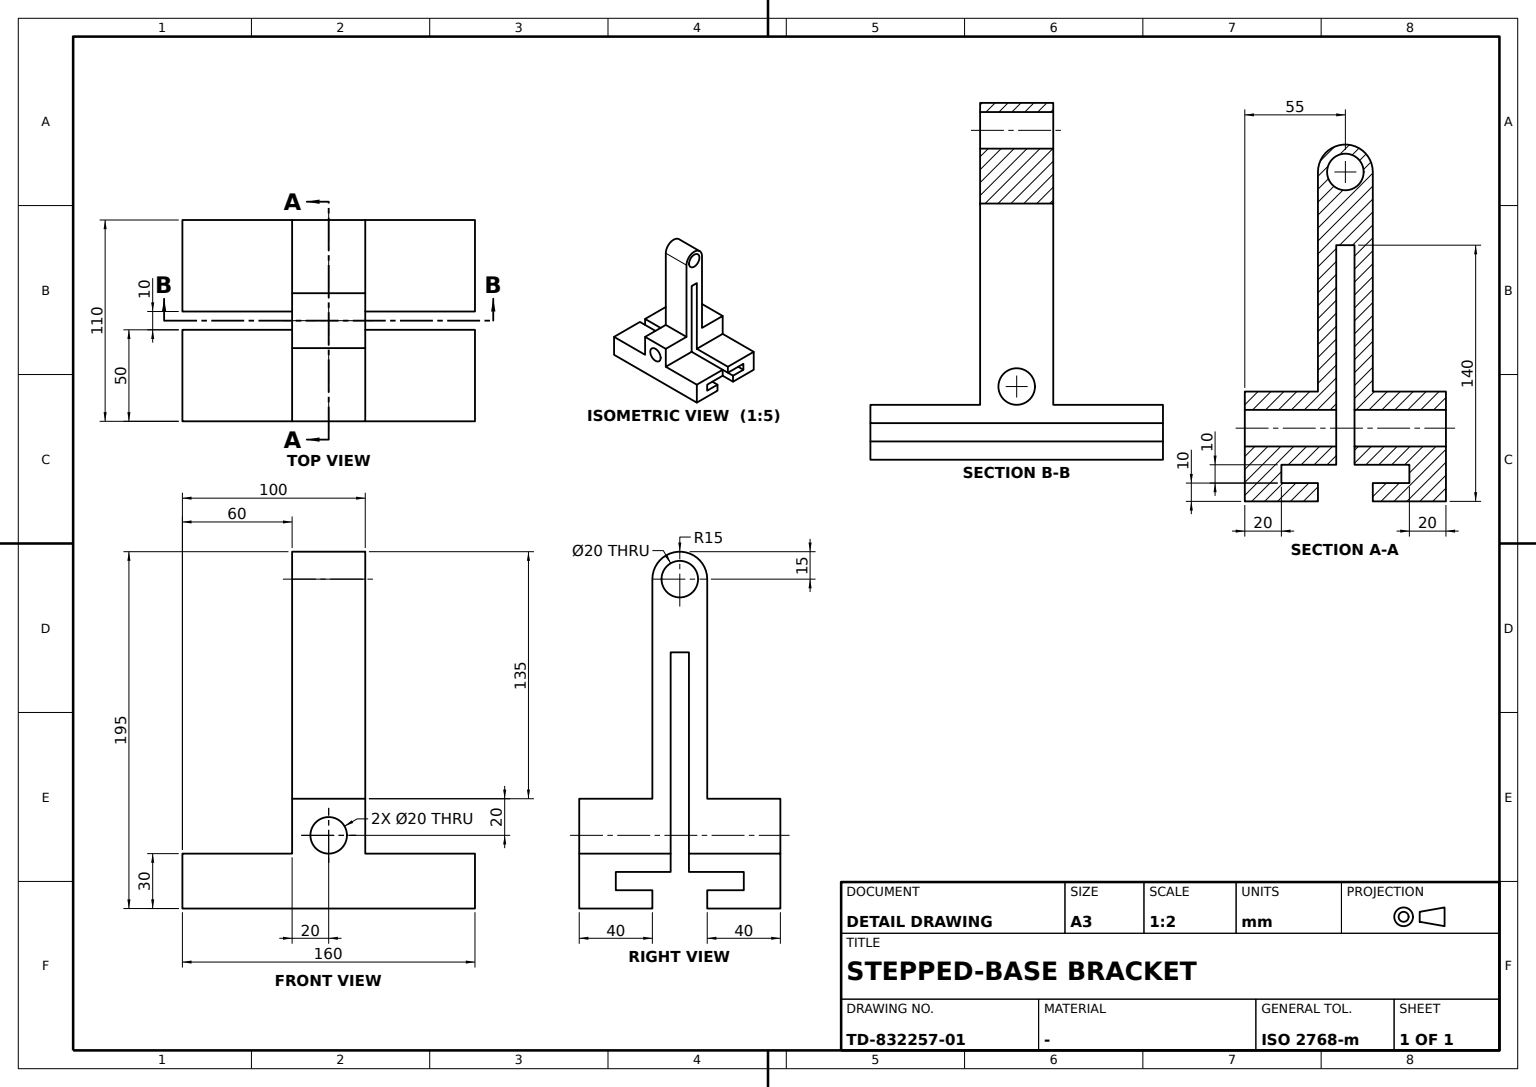
CATIA V5 part; units mm, degrees
sketch "Sketch1" plane through (0, 0, 0) normal (1, 0, 0) x (0, 1, 0)
  point P0 (-5, 0)
  line L0 (-5, 0) -> (-55, 0)
  point P1 (-55, 0)
  line L1 (-55, 0) -> (-55, -30)
  point P2 (-55, -30)
  line L2 (-55, -30) -> (-15, -30)
  point P3 (-15, -30)
  line L3 (-15, -30) -> (-15, -20)
  point P4 (-15, -20)
  line L4 (-15, -20) -> (-35, -20)
  point P5 (-35, -20)
  line L5 (-35, -20) -> (-35, -10)
  point P6 (-35, -10)
  line L6 (-35, -10) -> (-5, -10)
  point P7 (-5, -10)
  line L7 (-5, -10) -> (-5, 0)
  point P8 (5, 0)
  point P9 (55, 0)
  point P10 (55, -30)
  point P11 (15, -30)
  point P12 (15, -20)
  point P13 (35, -20)
  point P14 (35, -10)
  point P15 (5, -10)
  line L8 (5, 0) -> (55, 0)
  line L9 (55, 0) -> (55, -30)
  line L10 (55, -30) -> (15, -30)
  line L11 (15, -30) -> (15, -20)
  line L12 (15, -20) -> (35, -20)
  line L13 (35, -20) -> (35, -10)
  line L14 (35, -10) -> (5, -10)
  line L15 (5, -10) -> (5, 0)
  dimension "distance L7 L15" = 10
  dimension "distance L1 L9" = 110
  dimension "distance L1 L3" = 40
  dimension "distance L5 L3" = 20
  dimension "distance L0 L2" = 30
  dimension "distance L6 L4" = 10
  dimension "distance L14 x axis" = 10
  constraint coincidence P0 x-axis
  constraint horizontal L0 x-axis
  constraint horizontal L2 x-axis
  constraint horizontal L4 x-axis
  constraint horizontal L6 x-axis
  constraint vertical L1 y-axis
  constraint vertical L3 y-axis
  constraint vertical L5 y-axis
  constraint vertical L7 y-axis
  constraint symmetry P0 P8 y-axis
  constraint symmetry P1 P9 y-axis
  constraint symmetry P2 P10 y-axis
  constraint symmetry P3 P11 y-axis
  constraint symmetry P4 P12 y-axis
  constraint symmetry P5 P13 y-axis
  constraint symmetry P6 P14 y-axis
  constraint symmetry P7 P15 y-axis
  constraint symmetry L0 L8 y-axis
  constraint symmetry L1 L9 y-axis
  constraint symmetry L2 L10 y-axis
  constraint symmetry L3 L11 y-axis
  constraint symmetry L4 L12 y-axis
  constraint symmetry L5 L13 y-axis
  constraint symmetry L6 L14 y-axis
  constraint symmetry L7 L15 y-axis
extrude "Pad1" add sketch "Sketch1" along normal mid plane 160
sketch "Sketch2" plane through (0, 0, 0) normal (1, 0, 0) x (0, 1, 0)
  line L0 (-5, 0) -> (-55, 0)
  line L1 (55, 0) -> (5, 0)
  line L2 (55, 0) -> (55, 30)
  point P0 (-55, 30)
  line L3 (-55, 30) -> (-55, 0)
  line L4 (-5, 0) -> (-5, 110)
  line L5 (-5, 110) -> (5, 110)
  line L6 (5, 110) -> (5, 0)
  line L7 (-55, 30) -> (-15, 30)
  point P1 (-15, 30)
  arc A0 (15, 150) -> (-15, 150) centre (0, 150) ccw
  point P2 (0, 150)
  point P3 (-15, 30)
  line L8 (-15, 30) -> (-15, 150)
  point P4 (-15, 150)
  point P5 (15, 150)
  point P6 (15, 30)
  line L9 (15, 30) -> (15, 150)
  point P7 (15, 30)
  point P8 (55, 30)
  line L10 (55, 30) -> (15, 30)
  circle A1 centre (0, 150) radius 10
  point P9 (5, 141.3397)
  dimension "length L3" = 30
  dimension "distance P2 L7" = 120
  dimension "radius A0" = 15
  dimension "distance L5 L1" = 110
  dimension "radius A1" = 10
  constraint vertical L2 y-axis
  constraint vertical L3 y-axis
  constraint vertical L4 y-axis
  constraint vertical L6 y-axis
  constraint vertical L8 y-axis
  constraint horizontal L5 x-axis
  constraint horizontal L7 x-axis
  constraint equal size L3 L2
  constraint coincidence P2 y-axis
  constraint coincidence P1 P3
  constraint coincidence A1 P9
  constraint coincidence P9 L6
  constraint tangency L8 A0
  constraint symmetry P4 P5 y-axis
  constraint symmetry P3 P6 y-axis
  constraint symmetry L8 L9 y-axis
  constraint symmetry P1 P7 y-axis
  constraint symmetry P0 P8 y-axis
  constraint symmetry L7 L10 y-axis
extrude "Pad2" add sketch "Sketch2" along normal mid plane 40
sketch "Sketch3" plane through (0, 55, 0) normal (0, 1, 0) x (-1, 0, 0)
  circle A0 centre (0, 10) radius 10
  point P0 (0, 10)
  line L0 (20, 30) -> (-20, 30) construction
  dimension "radius A0" = 10
  dimension "distance P0 L0" = 20
  constraint coincidence P0 y-axis
extrude "Pocket1" cut sketch "Sketch3" against normal through all
properties part number "Mechanical Mounting Bracket with Vertical Slotted Support, Rounded Top Boss, and Stepped Base in CATIA"
